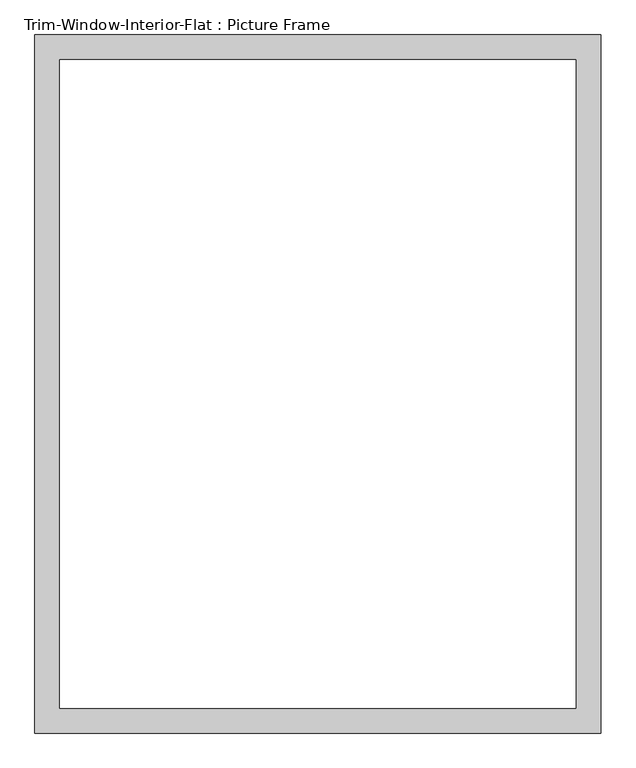
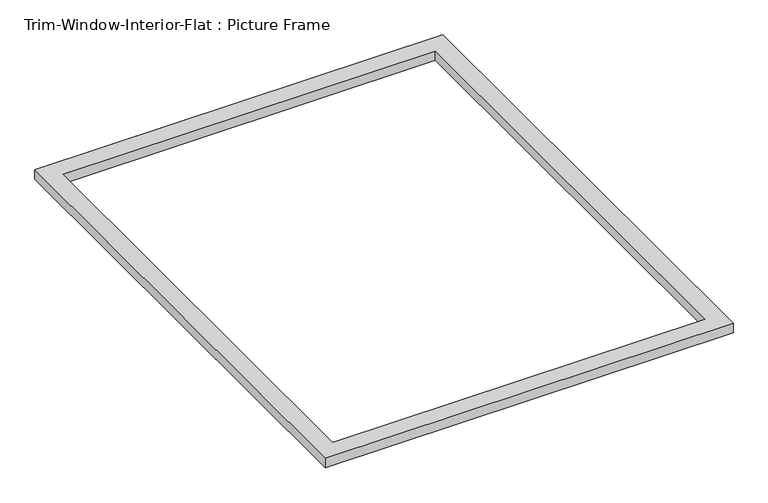
"""IFC4 building model written with IfcOpenShell, lengths in millimetres: proxy geometry, Trim-Window-Interior-Flat : Picture Frame."""

from ifc_helpers import new_model, si_unit, origin, origin_with_axes, place, context, project, spatial, polyline, outline, extrude, source, transform, mapped, element, save


def trim_window_interior_flat_picture_frame_3bb882cf(model_context):
    return source(origin(), model_context, "Body", "SweptSolid", [
        extrude(outline(polyline([(654.05, 44.45), (654.05, -1568.45), (-654.05, -1568.45), (-654.05, 44.45), (654.05, 44.45)]), holes=[polyline([(596.9, -12.7), (-596.9, -12.7), (-596.9, -1511.3), (596.9, -1511.3), (596.9, -12.7)])]), origin_with_axes(), (0.0, 0.0, 1.0), 31.75),
    ])


if __name__ == "__main__":
    model = new_model("IFC4")
    model_context = context("Model", 3, world=origin())
    ifc_project = project(units=[si_unit("LENGTHUNIT", "METRE", prefix="MILLI")], contexts=[model_context])
    site = spatial("IfcSite", under=ifc_project)
    building = spatial("IfcBuilding", under=site)
    placement = place(None, origin())
    trim_window_interior_flat_picture_frame_shape = trim_window_interior_flat_picture_frame_3bb882cf(model_context)
    element("IfcBuildingElementProxy", 1, Name="Trim-Window-Interior-Flat : Picture Frame", ObjectType="Trim-Window-Interior-Flat : Picture Frame", at=placement, inside=building, context=model_context, shape_type="MappedRepresentation", body=[
        mapped(trim_window_interior_flat_picture_frame_shape, transform((0.0, 0.0, 0.0), x_axis=(1.0, 0.0, 0.0), y_axis=(0.0, 1.0, 0.0), z_axis=(0.0, 0.0, 1.0))),
    ])
    save(model, "model.ifc")

# Revit data of these elements
# Type "Trim-Window-Interior-Flat : Picture Frame"
#   Trim Thickness_Picture Frame = 0' - 1 1/4"
#   Trim Width = 0' - 2 1/4"
#   Trim Thickness_with Sill = 0' - 0 3/4"
#   Sill Thickness = 0' - 1 1/4"
#   Opening Width [instance default] = 2' - 0"
#   Opening Height [instance default] = 3' - 0"
#   Default Elevation = 4' - 0"
#   Sill = no
#   Picture Frame = yes
#   Trim Material [instance default] = none
# Element 1 (IfcBuildingElementProxy, "Trim-Window-Interior-Flat : Picture Frame")
#   Opening Width = 4' - 0"
#   Opening Height = 5' - 0"
#   Trim Material = Wood - Stained
#   Materials on its faces: "Wood - Stained"
# Materials
#   "Wood - Stained": class "Wood", colour RGB 224 178 126, transparency 0, Cost = 0
